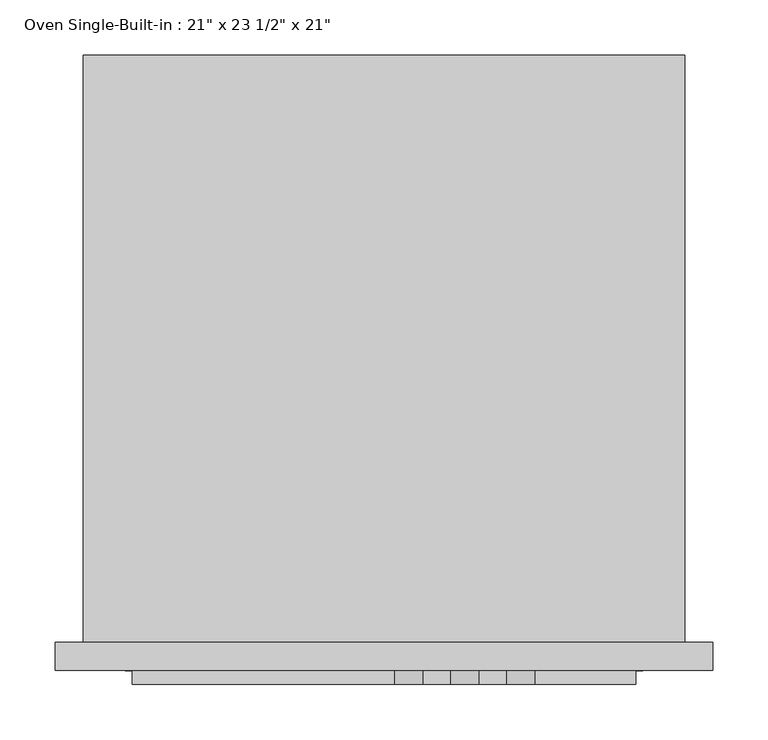
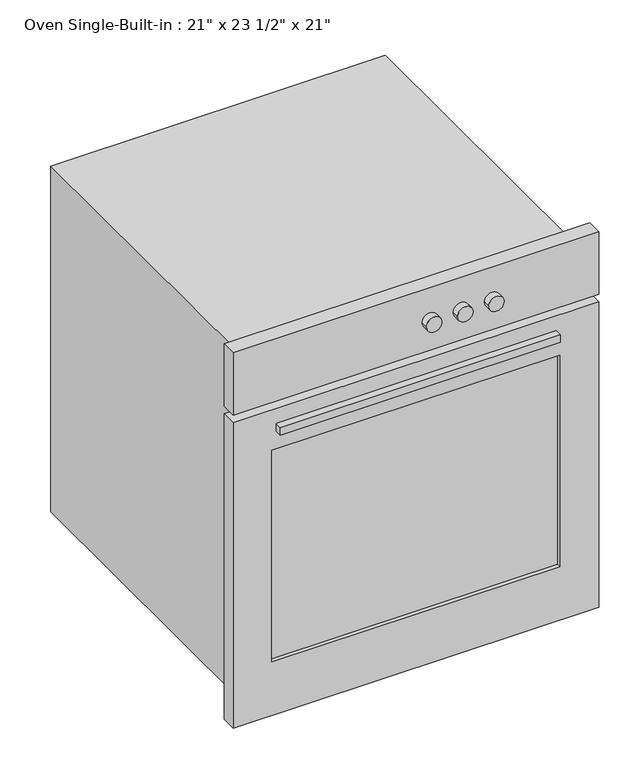
"""IFC4 building model written with IfcOpenShell, lengths in millimetres: proxy geometry."""

from ifc_helpers import new_model, si_unit, point, frame, frame_2d, origin, place, context, project, spatial, polyline, circle_curve, trimmed, segment, composite_curve, outline, extrude, faceted_brep, source, transform, mapped, element, save


def proxy_68898770(model_context):
    return source(origin(), model_context, "Body", "SolidModel", [
        extrude(outline(polyline([(263.2750727, -151.0341411), (-333.6249273, -151.0341411), (-333.6249273, -125.6341411), (263.2750727, -125.6341411), (263.2750727, -151.0341411)])), frame((0.0, 0.0, 755.65), z_axis=(0.0, 0.0, 1.0), x_axis=(1.0, 0.0, 0.0)), (0.0, 0.0, 1.0), 107.95),
        extrude(outline(polyline([(742.95, 263.2750727), (742.95, -333.6249273), (215.9, -333.6249273), (215.9, 263.2750727), (742.95, 263.2750727)]), holes=[polyline([(673.1, 199.7750727), (307.975, 199.7750727), (307.975, -270.1249273), (673.1, -270.1249273), (673.1, 199.7750727)])]), frame((0.0, -151.0341411, 0.0), z_axis=(0.0, 1.0, 0.0), x_axis=(0.0, 0.0, 1.0)), (0.0, 0.0, 1.0), 25.4),
        extrude(outline(polyline([(199.7750727, -144.6841411), (-270.1249273, -144.6841411), (-270.1249273, -138.3341411), (199.7750727, -138.3341411), (199.7750727, -144.6841411)])), frame((0.0, 0.0, 307.975), z_axis=(0.0, 0.0, 1.0), x_axis=(1.0, 0.0, 0.0)), (0.0, 0.0, 1.0), 365.125),
        extrude(outline(composite_curve([segment(trimmed(circle_curve(frame_2d((807.921693, -12.6998447)), 12.7), [point((807.921693, -25.3998447))], [point((807.921693, 0.0001553))], False, "CARTESIAN"), True, "CONTINUOUS"), segment(trimmed(circle_curve(frame_2d((807.921693, -12.6998447)), 12.7), [point((807.921693, 0.0001553))], [point((807.921693, -25.3998447))], False, "CARTESIAN"), True, "CONTINUOUS")], self_intersect=False)), frame((0.0, -163.7341411, 0.0), z_axis=(0.0, 1.0, 0.0), x_axis=(0.0, 0.0, 1.0)), (0.0, 0.0, 1.0), 12.7),
        extrude(outline(composite_curve([segment(trimmed(circle_curve(frame_2d((807.921693, 38.1001553)), 12.7), [point((807.921693, 25.4001553))], [point((807.921693, 50.8001553))], False, "CARTESIAN"), True, "CONTINUOUS"), segment(trimmed(circle_curve(frame_2d((807.921693, 38.1001553)), 12.7), [point((807.921693, 50.8001553))], [point((807.921693, 25.4001553))], False, "CARTESIAN"), True, "CONTINUOUS")], self_intersect=False)), frame((0.0, -163.7341411, 0.0), z_axis=(0.0, 1.0, 0.0), x_axis=(0.0, 0.0, 1.0)), (0.0, 0.0, 1.0), 12.7),
        extrude(outline(composite_curve([segment(trimmed(circle_curve(frame_2d((807.921693, 88.9001553)), 12.7), [point((807.921693, 76.2001553))], [point((807.921693, 101.6001553))], False, "CARTESIAN"), True, "CONTINUOUS"), segment(trimmed(circle_curve(frame_2d((807.921693, 88.9001553)), 12.7), [point((807.921693, 101.6001553))], [point((807.921693, 76.2001553))], False, "CARTESIAN"), True, "CONTINUOUS")], self_intersect=False)), frame((0.0, -163.7341411, 0.0), z_axis=(0.0, 1.0, 0.0), x_axis=(0.0, 0.0, 1.0)), (0.0, 0.0, 1.0), 12.7),
        extrude(outline(polyline([(193.4250727, -163.7341411), (-263.7749273, -163.7341411), (-263.7749273, -151.0341411), (193.4250727, -151.0341411), (193.4250727, -163.7341411)])), frame((0.0, 0.0, 704.9220137), z_axis=(0.0, 0.0, 1.0), x_axis=(1.0, 0.0, 0.0)), (0.0, 0.0, 1.0), 12.7),
        extrude(outline(polyline([(212.4750727, -125.6341411), (-282.8249273, -125.6341411), (-282.8249273, -100.2341411), (212.4750727, -100.2341411), (212.4750727, -125.6341411)])), frame((0.0, 0.0, 717.6220137), z_axis=(0.0, 0.0, 1.0), x_axis=(1.0, 0.0, 0.0)), (0.0, 0.0, 1.0), 95.1779863),
        faceted_brep([(237.8750727, -125.6341411, 838.2), (-308.2249273, -125.6341411, 838.2), (-308.2249273, -125.6341411, 241.3), (237.8750727, -125.6341411, 241.3), (212.4750727, -125.6341411, 812.8), (212.4750727, -125.6341411, 266.7), (-282.8249273, -125.6341411, 266.7), (-282.8249273, -125.6341411, 812.8), (237.8750727, 407.7658589, 838.2), (237.8750727, 407.7658589, 241.3), (-308.2249273, 407.7658589, 241.3), (-308.2249273, 407.7658589, 838.2), (212.4750727, 382.1090259, 812.8), (212.4750727, 382.1090259, 266.7), (-282.8249273, 382.1090259, 266.7), (-282.8249273, 382.1090259, 812.8)], [[[0, 1, 2, 3], [4, 5, 6, 7]], [[8, 9, 10, 11]], [[1, 0, 8, 11]], [[2, 1, 11, 10]], [[3, 2, 10, 9]], [[0, 3, 9, 8]], [[5, 4, 12, 13]], [[6, 5, 13, 14]], [[7, 6, 14, 15]], [[4, 7, 15, 12]], [[13, 12, 15, 14]]]),
    ])


if __name__ == "__main__":
    model = new_model("IFC4")
    model_context = context("Model", 3, world=origin())
    ifc_project = project(units=[si_unit("LENGTHUNIT", "METRE", prefix="MILLI")], contexts=[model_context])
    site = spatial("IfcSite", under=ifc_project)
    building = spatial("IfcBuilding", under=site)
    placement = place(None, origin())
    proxy_shape = proxy_68898770(model_context)
    element("IfcBuildingElementProxy", 1, Name="Oven Single-Built-in : 21\" x 23 1/2\" x 21\"", ObjectType="Oven Single-Built-in : 21\" x 23 1/2\" x 21\"", at=placement, inside=building, context=model_context, shape_type="MappedRepresentation", body=[
        mapped(proxy_shape, transform((0.0, 0.0, 0.0), x_axis=(1.0, 0.0, 0.0), y_axis=(0.0, 1.0, 0.0), z_axis=(0.0, 0.0, 1.0))),
    ])
    save(model, "model.ifc")

# Revit data of these elements
# Type "Oven Single-Built-in : 21\" x 23 1/2\" x 21\""
#   Label = "OVEN"
#   Assembly Code = "E1090400"
#   Depth = 1' - 9"
#   Height = 1' - 11 1/2"
#   Install Height = 0' - 9 1/2"
#   Width = 1' - 9 1/2"
#   Oven Material = Metal - Stainless Steel, Polished
#   Default Elevation = 0
# Element 1 (IfcBuildingElementProxy, "Oven Single-Built-in : 21\" x 23 1/2\" x 21\"")
#   Materials on its faces: "Metal - Steel", "Metal - Stainless Steel, Polished", "Glass"
# Materials
#   "Metal - Stainless Steel, Polished": colour RGB 215 215 215, transparency 0
#   "Metal - Steel": colour RGB 247 247 247, transparency 0
#   "Glass": class "Glass", colour RGB 0 128 192, transparency 0.75, Description = "Soda Lime Glass", Cost = 0
